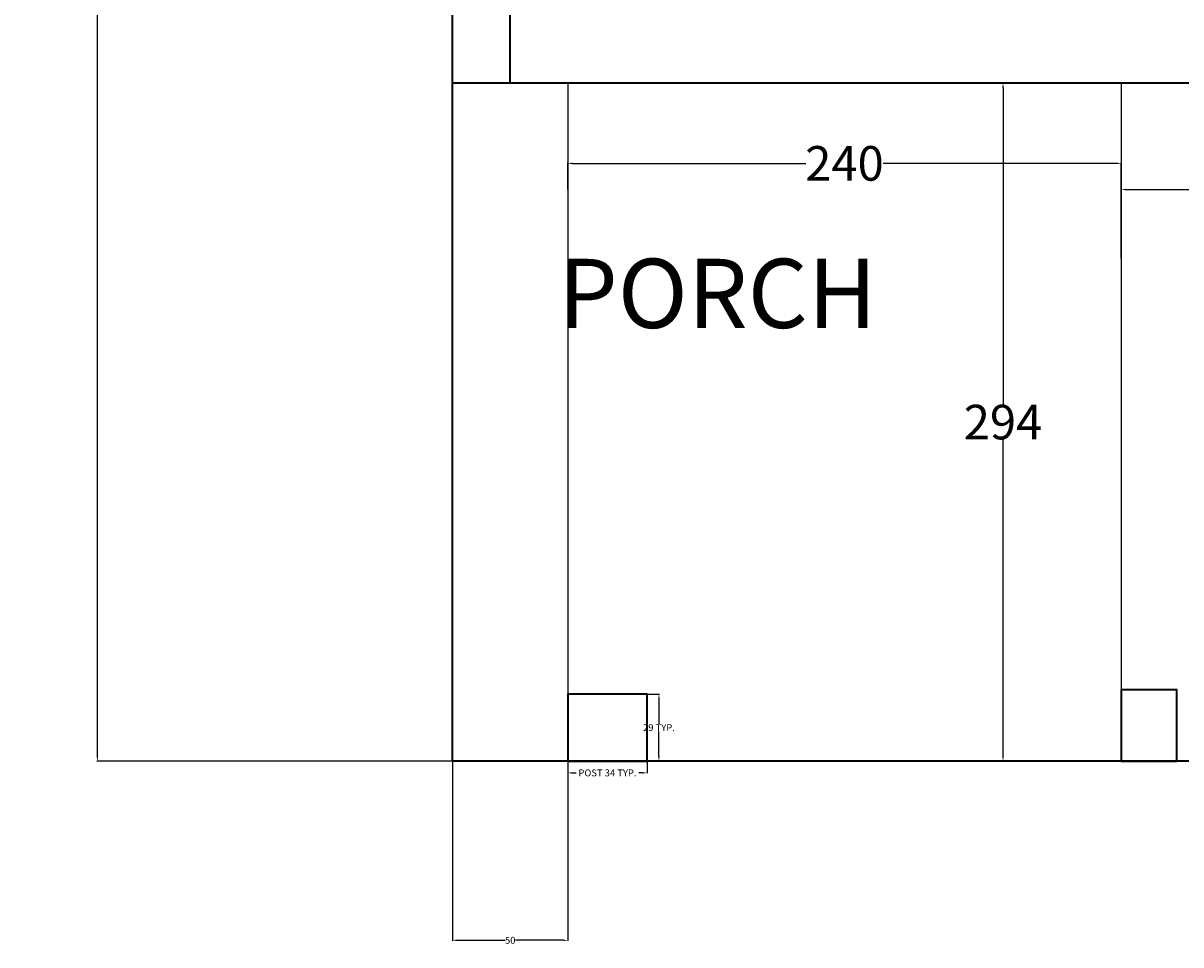
# Model space of a CAD drawing. Units: centimetres. Extents: x -121 to 3851, y -16 to 1180.
# Tile 1 of 16: x -121 to 381, y -16 to 384. Entities that reach past the tile are written whole.
import ezdxf

# ---------------------------------------------------------------- set-up
doc = ezdxf.new("R2010")
doc.units = ezdxf.units.CM
doc.header["$MEASUREMENT"] = 0
for name, color, linetype, lineweight in [('A-ANNO-DIMS', 2, 'Continuous', 18), ('A-AREA-IDEN', 3, 'Continuous', 18), ('A-COLS', 7, 'Continuous', 35), ('A-FLOR', 8, 'Continuous', 25), ('A-WALL', 7, 'Continuous', 35)]:
    doc.layers.add(name, color=color, linetype=linetype, lineweight=lineweight)
doc.styles.get("Standard").update_dxf_attribs({"font": 'arial.ttf'})
doc.dimstyles.get("Standard").update_dxf_attribs({"dimtxt": 3, "dimasz": 2, "dimexe": 0.18, "dimexo": 0.0625, "dimgap": 0.09, "dimtad": 0, "dimtih": 1, "dimtoh": 1, "dimdec": 0, "dimzin": 0, "dimdsep": 46, "dimtxsty": 'Standard', "dimcen": 0.09, "dimadec": 0, "dimazin": 0, "dimtfac": 1, "dimtdec": 0, "dimtofl": 0, "dimtmove": 0, "dimatfit": 3, "dimfxl": 1, "dimtolj": 1, "dimtzin": 0, "dimarcsym": 0})

# ---------------------------------------------------------------- blocks, each defined once
blk = doc.blocks.new('*D2')
at = {"layer": 'A-ANNO-DIMS', "color": 0, "lineweight": -2, "transparency": 16777216}
for p, q in [((64.98, 880.01), (-89.22, 880.01)), ((-89.04, 878.01), (-89.04, 487.42)), ((-89.04, 66.01), (-89.04, 456.61)), ((64.98, 64.01), (-89.22, 64.01))]:
    blk.add_line(p, q, dxfattribs=at)
at = {"layer": 'A-ANNO-DIMS', "color": 0, "transparency": 16777216}
for points in [[(-89.37, 878.01), (-88.71, 878.01), (-89.04, 880.01)], [(-89.37, 66.01), (-88.71, 66.01), (-89.04, 64.01)]]:
    blk.add_solid(points, dxfattribs=at)
at = {"layer": 'Defpoints', "color": 0, "transparency": 16777216}
for p in [(65.04, 880.01), (-89.04, 64.01), (65.04, 64.01)]:
    blk.add_point(p, dxfattribs=at)
at = {"layer": 'A-ANNO-DIMS', "color": 0, "transparency": 16777216, "insert": (-89.04, 472.01), "char_height": 3, "attachment_point": 5}
blk.add_mtext('\\A1;{\\H10x;816}', dxfattribs=at)
blk = doc.blocks.new('*D7')
at = {"layer": 'A-ANNO-DIMS', "color": 0, "lineweight": -2, "transparency": 16777216}
for p, q in [((291.28, 358.01), (303.97, 358.01)), ((303.79, 356.01), (303.79, 218.76)), ((303.79, 66.01), (303.79, 203.27)), ((291.28, 64.01), (303.97, 64.01))]:
    blk.add_line(p, q, dxfattribs=at)
at = {"layer": 'A-ANNO-DIMS', "color": 0, "transparency": 16777216}
for points in [[(303.45, 356.01), (304.12, 356.01), (303.79, 358.01)], [(303.45, 66.01), (304.12, 66.01), (303.79, 64.01)]]:
    blk.add_solid(points, dxfattribs=at)
at = {"layer": 'Defpoints', "color": 0, "transparency": 16777216}
for p in [(291.22, 358.01), (291.22, 64.01), (303.79, 64.01)]:
    blk.add_point(p, dxfattribs=at)
at = {"layer": 'A-ANNO-DIMS', "color": 0, "transparency": 16777216, "insert": (303.79, 211.01), "char_height": 3, "attachment_point": 5}
blk.add_mtext('\\A1;{\\H5x;294}', dxfattribs=at)
blk = doc.blocks.new('*D8')
at = {"layer": 'A-ANNO-DIMS', "color": 0, "lineweight": -2, "transparency": 16777216}
for p, q in [((355.04, 281.89), (355.04, 312.04)), ((357.04, 311.86), (393.83, 311.86)), ((473.04, 311.86), (436.25, 311.86)), ((475.04, 281.89), (475.04, 312.04))]:
    blk.add_line(p, q, dxfattribs=at)
at = {"layer": 'A-ANNO-DIMS', "color": 0, "transparency": 16777216}
for points in [[(357.04, 312.19), (357.04, 311.52), (355.04, 311.86)], [(473.04, 312.19), (473.04, 311.52), (475.04, 311.86)]]:
    blk.add_solid(points, dxfattribs=at)
at = {"layer": 'Defpoints', "color": 0, "transparency": 16777216}
for p in [(475.04, 311.86), (355.04, 281.82), (475.04, 281.82)]:
    blk.add_point(p, dxfattribs=at)
at = {"layer": 'A-ANNO-DIMS', "color": 0, "transparency": 16777216, "insert": (415.04, 311.86), "char_height": 3, "attachment_point": 5}
blk.add_mtext('\\A1;{\\H6.66667x;120}', dxfattribs=at)
blk = doc.blocks.new('*D9')
at = {"layer": 'A-ANNO-DIMS', "color": 0, "lineweight": -2, "transparency": 16777216}
for p, q in [((115.04, 311.92), (115.04, 323.39)), ((117.04, 323.21), (218.28, 323.21)), ((353.04, 323.21), (251.8, 323.21)), ((355.04, 311.92), (355.04, 323.39))]:
    blk.add_line(p, q, dxfattribs=at)
at = {"layer": 'A-ANNO-DIMS', "color": 0, "transparency": 16777216}
for points in [[(117.04, 323.54), (117.04, 322.88), (115.04, 323.21)], [(353.04, 323.54), (353.04, 322.88), (355.04, 323.21)]]:
    blk.add_solid(points, dxfattribs=at)
at = {"layer": 'Defpoints', "color": 0, "transparency": 16777216}
for p in [(115.04, 323.21), (115.04, 311.86), (355.04, 311.86)]:
    blk.add_point(p, dxfattribs=at)
at = {"layer": 'A-ANNO-DIMS', "color": 0, "transparency": 16777216, "insert": (235.04, 323.21), "char_height": 3, "attachment_point": 5}
blk.add_mtext('\\A1;{\\H5x;240}', dxfattribs=at)
blk = doc.blocks.new('POST-24X31CM')
blk.add_lwpolyline([(0, 0), (24.1, 0), (24.1, 30.82), (0, 30.82)], close=True)
blk = doc.blocks.new('POST-34X29CM')
blk.add_lwpolyline([(0, 0), (34.36, 0), (34.36, 28.96), (0, 28.96)], close=True)
blk = doc.blocks.new('*D37')
at = {"layer": 'A-ANNO-DIMS', "color": 0, "lineweight": -2, "transparency": 16777216}
for p, q in [((115.04, 63.95), (115.04, 58.68)), ((149.4, 63.95), (149.4, 58.68)), ((117.04, 58.86), (118.61, 58.86)), ((147.4, 58.86), (145.82, 58.86))]:
    blk.add_line(p, q, dxfattribs=at)
at = {"layer": 'A-ANNO-DIMS', "color": 0, "transparency": 16777216}
for points in [[(117.04, 59.19), (117.04, 58.53), (115.04, 58.86)], [(147.4, 59.19), (147.4, 58.53), (149.4, 58.86)]]:
    blk.add_solid(points, dxfattribs=at)
at = {"layer": 'Defpoints', "color": 0, "transparency": 16777216}
for p in [(115.04, 64.01), (149.4, 64.01), (149.4, 58.86)]:
    blk.add_point(p, dxfattribs=at)
at = {"layer": 'A-ANNO-DIMS', "color": 0, "transparency": 16777216, "insert": (132.22, 58.86), "char_height": 3, "attachment_point": 5}
blk.add_mtext('\\A1;POST 34 TYP.', dxfattribs=at)
blk = doc.blocks.new('*D38')
at = {"layer": 'A-ANNO-DIMS', "color": 0, "lineweight": -2, "transparency": 16777216}
for p, q in [((149.46, 92.97), (154.73, 92.97)), ((154.55, 90.97), (154.55, 80.11)), ((154.55, 66.01), (154.55, 76.87)), ((149.46, 64.01), (154.73, 64.01))]:
    blk.add_line(p, q, dxfattribs=at)
at = {"layer": 'A-ANNO-DIMS', "color": 0, "transparency": 16777216}
for points in [[(154.22, 90.97), (154.89, 90.97), (154.55, 92.97)], [(154.22, 66.01), (154.89, 66.01), (154.55, 64.01)]]:
    blk.add_solid(points, dxfattribs=at)
at = {"layer": 'Defpoints', "color": 0, "transparency": 16777216}
for p in [(149.4, 92.97), (154.55, 92.97), (149.4, 64.01)]:
    blk.add_point(p, dxfattribs=at)
at = {"layer": 'A-ANNO-DIMS', "color": 0, "transparency": 16777216, "insert": (154.55, 78.49), "char_height": 3, "attachment_point": 5}
blk.add_mtext('\\A1;29 TYP.', dxfattribs=at)
blk = doc.blocks.new('*D55')
at = {"layer": 'A-ANNO-DIMS', "color": 0, "lineweight": -2, "transparency": 16777216}
for p, q in [((65.04, 63.95), (65.04, -13.92)), ((115.04, 63.95), (115.04, -13.92)), ((67.04, -13.74), (87.8, -13.74)), ((113.04, -13.74), (92.27, -13.74))]:
    blk.add_line(p, q, dxfattribs=at)
at = {"layer": 'A-ANNO-DIMS', "color": 0, "transparency": 16777216}
for points in [[(67.04, -13.4), (67.04, -14.07), (65.04, -13.74)], [(113.04, -13.4), (113.04, -14.07), (115.04, -13.74)]]:
    blk.add_solid(points, dxfattribs=at)
at = {"layer": 'Defpoints', "color": 0, "transparency": 16777216}
for p in [(65.04, 64.01), (115.04, 64.01), (115.04, -13.74)]:
    blk.add_point(p, dxfattribs=at)
at = {"layer": 'A-ANNO-DIMS', "color": 0, "transparency": 16777216, "insert": (90.04, -13.74), "char_height": 3, "attachment_point": 5}
blk.add_mtext('\\A1;50', dxfattribs=at)

msp = doc.modelspace()

# ---------------------------------------------------------------- linework, layer by layer
at = {"layer": 'A-FLOR'}
for p, q in [((115.0382, 358.0141), (115.0382, 64.0141)), ((355.0382, 358.0141), (355.0382, 64.0141))]:
    msp.add_line(p, q, dxfattribs=at)
at = {"layer": 'A-WALL'}
for p, q in [((65.0382, 64.0141), (65.0382, 880.0141)), ((90.0382, 358.0141), (90.0382, 678.0141)), ((475.0382, 358.0141), (65.0382, 358.0141)), ((1421.0382, 64.0141), (65.0382, 64.0141))]:
    msp.add_line(p, q, dxfattribs=at)

# ---------------------------------------------------------------- block references
at = {"layer": 'A-COLS'}
for name, p in [('POST-34X29CM', (115.038, 64.014)), ('POST-24X31CM', (355.038, 64.014))]:
    msp.add_blockref(name, p, dxfattribs=at)

# ---------------------------------------------------------------- texts
at = {"layer": 'A-AREA-IDEN', "insert": (110.8008, 281.8249), "char_height": 30, "attachment_point": 1}
msp.add_mtext_dynamic_manual_height_columns('PORCH', width=127.068665, gutter_width=1, heights=[0], dxfattribs=at)

# ---------------------------------------------------------------- dimensions: what is measured, and where the dimension line sits
at = {"layer": 'A-ANNO-DIMS'}
for base, p1, p2, text, override, picture, middle in [((-89.041, 64.0141), (65.0382, 880.0141), (65.0382, 64.0141), '{\\H10x;<>}', {"dimclrd": 0, "dimclre": 0, "dimclrt": 0}, '*D2', (-89.041, 472.0141)), ((303.7867, 64.0141), (291.2218, 358.0141), (291.2218, 64.0141), '{\\H5x;<>}', {"dimclrd": 0, "dimclre": 0, "dimclrt": 0}, '*D7', (303.7867, 211.0141)), ((154.5523, 92.9694), (149.3983, 64.0141), (149.3983, 92.9694), '<> TYP.', {"dimdec": 0, "dimlfac": 1, "dimrnd": 0, "dimzin": 0, "dimdsep": 46, "dimlunit": 2}, '*D38', (154.5523, 78.4917))]:
    dim = msp.add_linear_dim(base=base, p1=p1, p2=p2, angle=90, text=text, dimstyle='Standard', override=override, dxfattribs=at)
    dim.commit()
    dim.dimension.update_dxf_attribs({"geometry": picture, "text_midpoint": middle})
for base, p1, p2, text, override, picture, middle in [((115.0382, 323.2094), (355.0382, 311.8567), (115.0382, 311.8567), '{\\H5x;<>}', {"dimclrd": 0, "dimclre": 0, "dimclrt": 0}, '*D9', (235.0382, 323.2094)), ((475.0382, 311.8567), (355.0382, 281.8249), (475.0382, 281.8249), '{\\H6.66667x;<>}', {"dimclrd": 0, "dimclre": 0, "dimclrt": 0}, '*D8', (415.0382, 311.8567)), ((149.3983, 58.8601), (115.0382, 64.0141), (149.3983, 64.0141), 'POST <> TYP.', {"dimdec": 0, "dimlfac": 1, "dimrnd": 0, "dimzin": 0, "dimdsep": 46, "dimlunit": 2}, '*D37', (132.2182, 58.8601))]:
    dim = msp.add_linear_dim(base=base, p1=p1, p2=p2, text=text, dimstyle='Standard', override=override, dxfattribs=at)
    dim.commit()
    dim.dimension.update_dxf_attribs({"geometry": picture, "text_midpoint": middle})
dim = msp.add_linear_dim(base=(115.0382, -13.7359), p1=(65.0382, 64.0141), p2=(115.0382, 64.0141), dimstyle='Standard', override={"dimdec": 0, "dimlfac": 1, "dimrnd": 0, "dimzin": 0, "dimdsep": 46, "dimlunit": 2}, dxfattribs=at)
dim.commit()
dim.dimension.update_dxf_attribs({"geometry": '*D55', "text_midpoint": (90.0382, -13.7359)})

doc.saveas('drawing.dxf')
